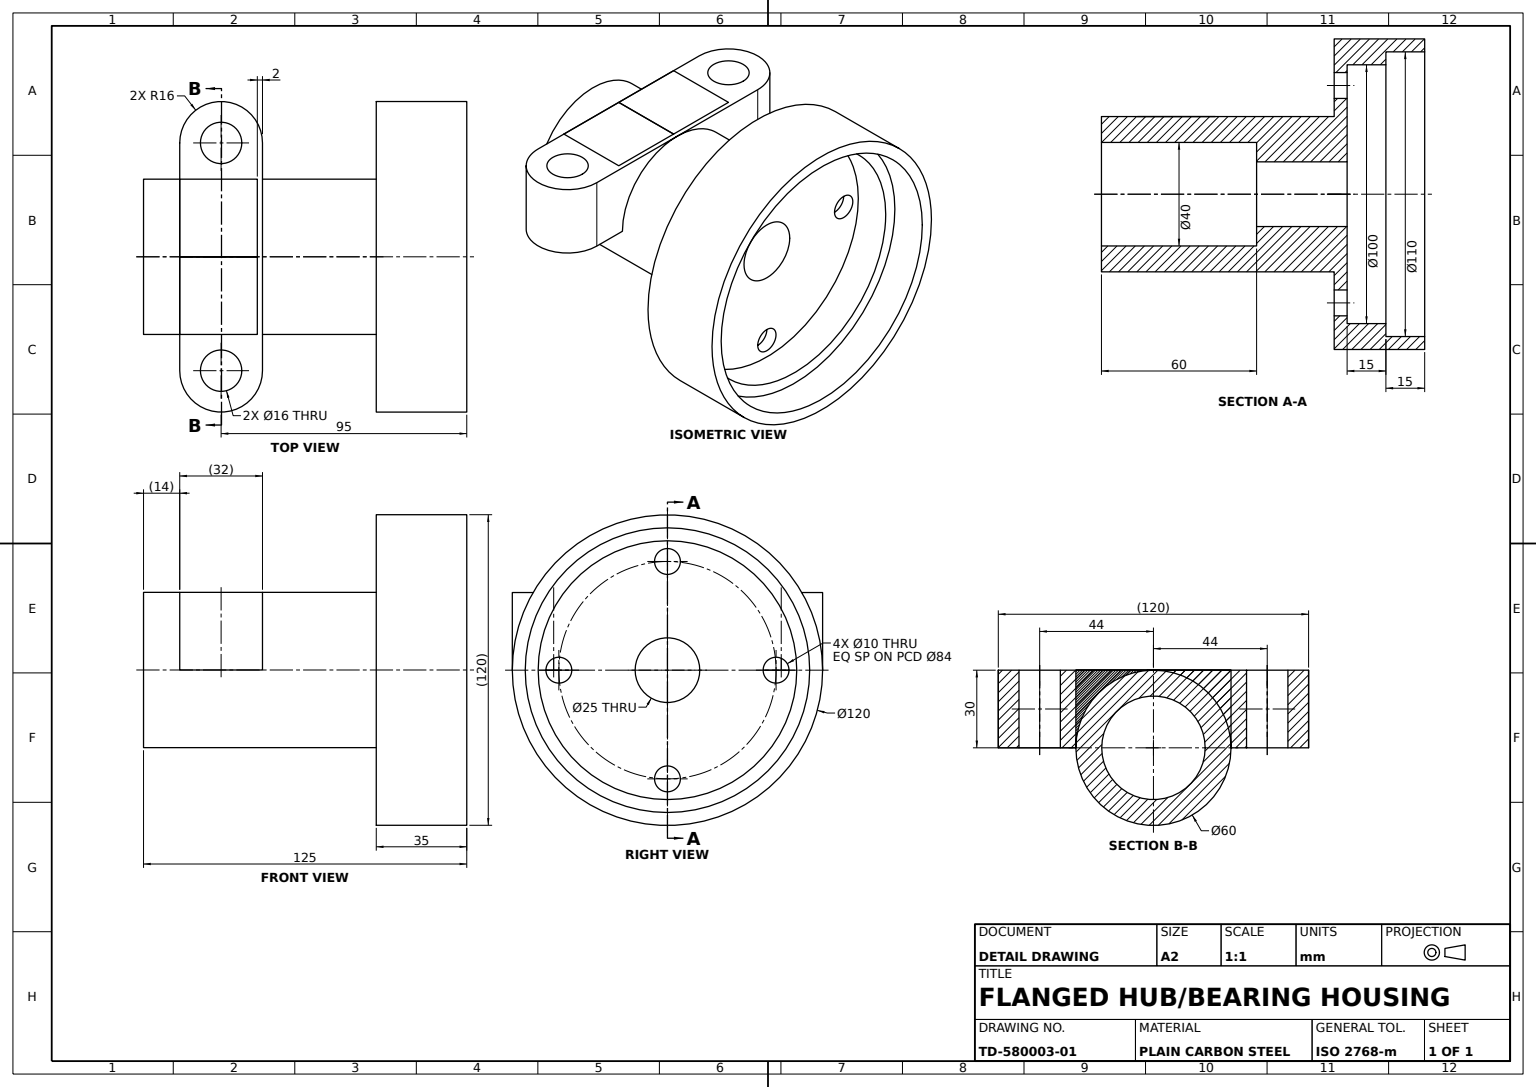
SolidWorks part; units mm, degrees
material "Plain Carbon Steel"
ref_plane "Front Plane" through (0, 0, 0) normal (0, 0, 1) x (1, 0, 0)
ref_plane "Top Plane" through (0, 0, 0) normal (0, 1, 0) x (1, 0, 0)
ref_plane "Right Plane" through (0, 0, 0) normal (1, 0, 0) x (0, 0, -1)
sketch "Flange Sketch Ø120" plane through (0, 0, 0) normal (0, 0, 1) x (1, 0, 0)
  circle A0 centre (0, 0) radius 60
  dimension "D1" = 120
extrude "Flange Ø120" add sketch "Flange Sketch Ø120" along normal blind 35
sketch "Flange Recess Sketch Ø110" plane through (0, 0, 0) normal (0, 0, -1) x (-1, 0, 0)
  circle A0 centre (0, 0) radius 55
  dimension "D1" = 110
extrude "Flange Recess Ø110" cut sketch "Flange Recess Sketch Ø110" against normal blind 15
sketch "Flange Inner Cut Sketch" plane through (0, 0, 15) normal (0, 0, -1) x (-1, 0, 0)
  circle A0 centre (0, 0) radius 50
  dimension "D1" = 100
extrude "Flange Inner Cut" cut sketch "Flange Inner Cut Sketch" against normal blind 15
sketch "Bolt Holes Sketch 4xØ10" plane through (0, 0, 35) normal (0, 0, 1) x (1, 0, 0)
  circle A0 centre (0, 0) radius 42 construction
  circle A1 centre (42, 0) radius 5
  circle A2 centre (0, -42) radius 5
  circle A3 centre (-42, 0) radius 5
  circle A4 centre (0, 42) radius 5
  dimension "D1" = 4
  dimension "D2" = 84
  dimension "D3" = 10
  dimension "D4" = 42
  dimension "D5" = 42
extrude "Bolt Holes 4xØ10" cut sketch "Bolt Holes Sketch 4xØ10" against normal blind 15
sketch "Hub Sketch Ø60" plane through (0, 0, 35) normal (0, 0, 1) x (1, 0, 0)
  circle A0 centre (0, 0) radius 30
  dimension "D1" = 60
extrude "Hub Ø60" add sketch "Hub Sketch Ø60" along normal blind 30
sketch "Hub Extension Sketch" plane through (0, 0, 65) normal (0, 0, 1) x (1, 0, 0)
  line L0 (-30, 0) -> (-20, 0)
  line L1 (20, 0) -> (30, 0)
  arc A0 (-30, 0) -> (30, 0) centre (0, 0) ccw
  arc A1 (-20, 0) -> (20, 0) centre (0, 0) ccw
  dimension "D1" = 60
  dimension "D2" = 40
extrude "Hub Extension" add sketch "Hub Extension Sketch" along normal blind 60
sketch "Clamp Lugs Sketch" plane through (0, 0, 0) normal (0, 1, 0) x (1, 0, 0)
  line L0 (44, -79) -> (30, -79)
  line L2 (30, -125) -> (30, -65) construction
  line L3 (30, -79) -> (30, -111)
  line L4 (30, -111) -> (44, -111)
  line L5 (-20, -125) -> (20, -125) construction
  line L7 (-30, -111) -> (-44, -111)
  line L8 (-30, -79) -> (-30, -111)
  line L9 (-44, -79) -> (-30, -79)
  arc A0 (44, -111) -> (44, -79) centre (44, -95) ccw
  circle A1 centre (44, -95) radius 8
  circle A2 centre (-44, -95) radius 8
  arc A3 (-44, -111) -> (-44, -79) centre (-44, -95) cw
  point P11 (0, -125)
  dimension "D1" = 16
  dimension "D2" = 16
  dimension "D6" = 16
  dimension "D7" = 16
  dimension "D3" = 14
  dimension "D4" = 95
  dimension "D5" = 95
  dimension "D8" = 32
  dimension "D9" = 14
  dimension "D10" = 44
  dimension "D11" = 60
  dimension "D12" = 32
extrude "Clamp Lugs" add sketch "Clamp Lugs Sketch" against normal blind 30 separate body
sketch "Lug Web A Sketch" plane through (0, 0, 111) normal (0, 0, 1) x (1, 0, 0)
  line L0 (30, -30) -> (30, 0)
  line L1 (0, -30) -> (30, -30)
  line L2 (-30, 0) -> (-30, -30)
  line L3 (-30, -30) -> (0, -30)
  arc A0 (-30, 0) -> (30, 0) centre (0, 0) ccw construction
  arc A1 (-30, 0) -> (30, 0) centre (0, 0) ccw
  line M3 (30, 0) -> (30, -30)
sketch "Shaft Bore Sketch" plane through (0, 0, 65) normal (0, 0, 1) x (1, 0, 0)
  circle A0 centre (0, 0) radius 12.5
  dimension "D1" = 25
extrude "Shaft Bore" cut sketch "Shaft Bore Sketch" against normal blind 113
sketch "Hub Tube Sketch Ø60-Ø40" plane through (0, 0, 125) normal (0, 0, 1) x (1, 0, 0)
  circle A0 centre (0, 0) radius 30
  circle A1 centre (0, 0) radius 20
  dimension "D1" = 60
  dimension "D2" = 40
extrude "Hub Tube" add sketch "Hub Tube Sketch Ø60-Ø40" against normal blind 60
sketch "Lug Web B Sketch" plane through (0, 0, 111) normal (0, 0, 1) x (1, 0, 0)
  line L0 (30, 0) -> (30, -30)
  line L1 (30, -30) -> (0, -30)
  line L2 (0, -30) -> (-30, -30)
  line L3 (-30, -30) -> (-30, 0)
  circle A0 centre (0, 0) radius 30 construction
  circle A1 centre (0, 0) radius 30 construction
  arc A2 (-30, 0) -> (30, 0) centre (0, 0) ccw
  line M3 (30, 0) -> (30, -30)
extrude "Lug Web B" add sketch "Lug Web B Sketch" against normal blind 32 contours A2 L1 M3 | A2 L3 L2
extrude "Lug Web A" add sketch "Lug Web A Sketch" against normal blind 30 separate body contours A1 L1 M3 | A1 L2 L3
